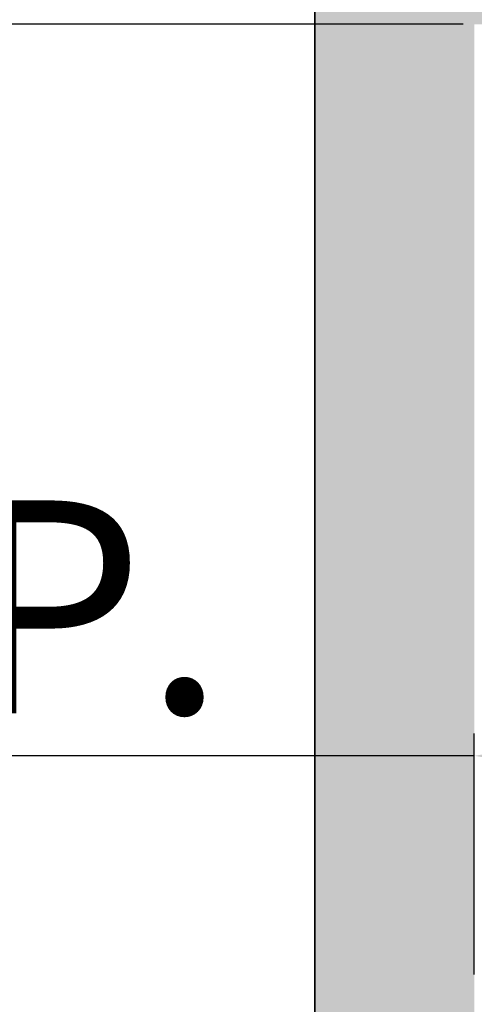
# Model space of a CAD drawing. Units: inches. Extents: x 2083 to 3317, y 1141 to 2115.
# Tile 11 of 256: x 2210 to 2236, y 1361 to 1417. Entities that reach past the tile are written whole.
import ezdxf

# ---------------------------------------------------------------- set-up
doc = ezdxf.new("R2010")
doc.units = ezdxf.units.IN
doc.layers.add('A-ANNO-DIMS', color=2, linetype='Continuous', lineweight=18)
doc.layers.add('A-WALL', color=7, linetype='Continuous', lineweight=35)
doc.layers.add('A-WALL-PATT', color=251, linetype='Continuous', lineweight=13, true_color=0x636466)
doc.styles.get("Standard").update_dxf_attribs({"font": 'arial.ttf'})
doc.dimstyles.new('ISO-25', dxfattribs={"dimtxt": 12, "dimasz": 12, "dimexe": 1.25, "dimexo": 0.625, "dimtad": 1, "dimlunit": 3, "dimtxsty": 'Standard', "dimcen": 2.5, "dimadec": 0, "dimazin": 0, "dimtfac": 1, "dimtmove": 0, "dimatfit": 3, "dimfxl": 1, "dimarcsym": 0})

# ---------------------------------------------------------------- blocks, each defined once
blk = doc.blocks.new('*D13')
at = {"layer": 'A-ANNO-DIMS', "color": 0, "lineweight": -2, "transparency": 16777216}
for p, q in [((2226.335, 1477.761), (2191.976, 1477.761)), ((2193.226, 1465.761), (2193.226, 1275.261)), ((2226.335, 1263.261), (2191.976, 1263.261))]:
    blk.add_line(p, q, dxfattribs=at)
at = {"layer": 'A-ANNO-DIMS', "color": 0, "transparency": 16777216}
for points in [[(2191.226, 1465.761), (2195.226, 1465.761), (2193.226, 1477.761)], [(2191.226, 1275.261), (2195.226, 1275.261), (2193.226, 1263.261)]]:
    blk.add_solid(points, dxfattribs=at)
at = {"layer": 'Defpoints', "color": 0, "transparency": 16777216}
for p in [(2226.96, 1477.761), (2193.226, 1263.261), (2226.96, 1263.261)]:
    blk.add_point(p, dxfattribs=at)
at = {"layer": 'A-ANNO-DIMS', "color": 0, "transparency": 16777216, "insert": (2186.474, 1370.511), "char_height": 12, "attachment_point": 5, "rotation": 90}
blk.add_mtext('17\'-10.5"', dxfattribs=at)
blk = doc.blocks.new('*D22')
at = {"layer": 'A-ANNO-DIMS', "color": 0, "lineweight": -2, "transparency": 16777216}
for p, q in [((2235.96, 1362.739), (2235.96, 1376.309)), ((2322.26, 1362.739), (2322.26, 1376.309)), ((2235.96, 1375.059), (2083.007, 1375.059)), ((2310.26, 1375.059), (2247.96, 1375.059))]:
    blk.add_line(p, q, dxfattribs=at)
at = {"layer": 'A-ANNO-DIMS', "color": 0, "transparency": 16777216}
for points in [[(2247.96, 1377.059), (2247.96, 1373.059), (2235.96, 1375.059)], [(2310.26, 1377.059), (2310.26, 1373.059), (2322.26, 1375.059)]]:
    blk.add_solid(points, dxfattribs=at)
at = {"layer": 'Defpoints', "color": 0, "transparency": 16777216}
for p in [(2235.96, 1375.059), (2235.96, 1362.114), (2322.26, 1362.114)]:
    blk.add_point(p, dxfattribs=at)
at = {"layer": 'A-ANNO-DIMS', "color": 0, "transparency": 16777216, "insert": (2153.483, 1381.889), "char_height": 12, "attachment_point": 5}
blk.add_mtext('BED 7\'-2 1/2" TYP.', dxfattribs=at)
blk = doc.blocks.new('*D30')
at = {"layer": 'A-ANNO-DIMS', "color": 0, "lineweight": -2, "transparency": 16777216}
for p, q in [((2240.018, 1445.274), (2240.018, 1448.046)), ((2254.329, 1445.274), (2254.329, 1448.046)), ((2228.018, 1446.796), (2216.018, 1446.796)), ((2240.018, 1446.796), (2254.329, 1446.796)), ((2266.329, 1446.796), (2413.765, 1446.796))]:
    blk.add_line(p, q, dxfattribs=at)
at = {"layer": 'A-ANNO-DIMS', "color": 0, "transparency": 16777216}
for points in [[(2228.018, 1448.796), (2228.018, 1444.796), (2240.018, 1446.796)], [(2266.329, 1448.796), (2266.329, 1444.796), (2254.329, 1446.796)]]:
    blk.add_solid(points, dxfattribs=at)
at = {"layer": 'Defpoints', "color": 0, "transparency": 16777216}
for p in [(2254.329, 1446.796), (2240.018, 1444.649), (2254.329, 1444.649)]:
    blk.add_point(p, dxfattribs=at)
at = {"layer": 'A-ANNO-DIMS', "color": 0, "transparency": 16777216, "insert": (2346.047, 1453.625), "char_height": 12, "attachment_point": 5}
blk.add_mtext('WC 1\'-2 1/2" TYP.', dxfattribs=at)
blk = doc.blocks.new('*D31')
at = {"layer": 'A-ANNO-DIMS', "color": 0, "lineweight": -2, "transparency": 16777216}
for p, q in [((2237.871, 1456.649), (2237.871, 1541.915)), ((2239.393, 1444.649), (2236.621, 1444.649)), ((2237.871, 1431.548), (2237.871, 1444.649)), ((2239.393, 1431.548), (2236.621, 1431.548)), ((2237.871, 1419.548), (2237.871, 1407.548))]:
    blk.add_line(p, q, dxfattribs=at)
at = {"layer": 'A-ANNO-DIMS', "color": 0, "transparency": 16777216}
for points in [[(2235.871, 1456.649), (2239.871, 1456.649), (2237.871, 1444.649)], [(2235.871, 1419.548), (2239.871, 1419.548), (2237.871, 1431.548)]]:
    blk.add_solid(points, dxfattribs=at)
at = {"layer": 'Defpoints', "color": 0, "transparency": 16777216}
for p in [(2237.871, 1444.649), (2240.018, 1444.649), (2240.018, 1431.548)]:
    blk.add_point(p, dxfattribs=at)
at = {"layer": 'A-ANNO-DIMS', "color": 0, "transparency": 16777216, "insert": (2231.217, 1505.282), "char_height": 12, "attachment_point": 5, "rotation": 90}
blk.add_mtext('1\'-1" TYP.', dxfattribs=at)
blk = doc.blocks.new('*D47')
at = {"layer": 'A-ANNO-DIMS', "color": 0, "lineweight": -2, "transparency": 16777216}
for p, q in [((2235.335, 1416.261), (2173.36, 1416.261)), ((2174.61, 1284.261), (2174.61, 1404.261)), ((2235.335, 1272.261), (2173.36, 1272.261))]:
    blk.add_line(p, q, dxfattribs=at)
at = {"layer": 'A-ANNO-DIMS', "color": 0, "transparency": 16777216}
for points in [[(2172.61, 1404.261), (2176.61, 1404.261), (2174.61, 1416.261)], [(2172.61, 1284.261), (2176.61, 1284.261), (2174.61, 1272.261)]]:
    blk.add_solid(points, dxfattribs=at)
at = {"layer": 'Defpoints', "color": 0, "transparency": 16777216}
for p in [(2174.61, 1416.261), (2235.96, 1416.261), (2235.96, 1272.261)]:
    blk.add_point(p, dxfattribs=at)
at = {"layer": 'A-ANNO-DIMS', "color": 0, "transparency": 16777216, "insert": (2167.858, 1344.261), "char_height": 12, "attachment_point": 5, "rotation": 90}
blk.add_mtext('12\'-0"', dxfattribs=at)

msp = doc.modelspace()

# ---------------------------------------------------------------- hatches: boundary and pattern name
at = {"layer": 'A-WALL-PATT'}
h = msp.add_hatch(color=256, dxfattribs=at)
h.dxf.hatch_style = 1
h.paths.add_polyline_path([(3126.96, 2020.761), (2748.96, 2020.761), (2604.96, 2020.761), (2226.96, 2020.761), (2226.96, 1702.761), (2466.96, 1702.761), (2466.96, 1582.761), (2418.96, 1582.761), (2418.96, 1477.761), (2226.96, 1477.761), (2226.96, 1263.261), (2544.96, 1263.261), (2544.96, 1411.761), (2604.96, 1411.761), (2685.96, 1411.761), (2685.96, 1420.761), (2604.96, 1420.761), (2604.96, 1573.761), (2604.96, 1702.761), (2604.96, 2011.761), (2748.96, 2011.761), (2748.96, 1702.761), (2862.96, 1702.761), (2862.96, 1621.761), (2871.96, 1621.761), (2871.96, 1702.761), (2883.96, 1702.761), (2883.96, 1706.939, -0.026459), (2883.96, 1711.761), (2757.96, 1711.761), (2757.96, 1807.761), (2787.96, 1807.761), (2787.96, 1812.261), (2757.96, 1812.261), (2757.96, 2011.761), (2877.96, 2011.761), (2877.96, 1812.261), (2847.96, 1812.261), (2847.96, 1807.761), (2889.836, 1807.761), (2889.836, 1812.261), (2882.46, 1812.261), (2882.46, 2011.761), (3117.96, 2011.761), (3117.96, 1812.261), (2937.836, 1812.261), (2937.836, 1807.761), (2995.71, 1807.761), (2995.71, 1796.118), (3000.21, 1796.118), (3000.21, 1807.761), (3117.96, 1807.761), (3117.96, 1711.761), (3000.21, 1711.761), (3000.21, 1760.118), (2998.573, 1760.118, -0.020711), (2995.71, 1760.118), (2995.71, 1711.761), (2931.96, 1711.761), (2931.96, 1702.761), (3126.96, 1702.761)])
h.paths.add_polyline_path([(2471.46, 2011.761), (2471.46, 1810.011), (2462.717, 1810.011), (2462.717, 1805.511), (2505.96, 1805.511), (2505.96, 1810.011), (2475.96, 1810.011), (2475.96, 2011.761), (2595.96, 2011.761), (2595.96, 1810.011), (2565.96, 1810.011), (2565.96, 1805.511), (2595.96, 1805.511), (2595.96, 1711.761), (2235.96, 1711.761), (2235.96, 1805.511), (2353.71, 1805.511), (2353.71, 1796.054), (2358.21, 1796.054), (2358.21, 1805.511), (2414.717, 1805.511), (2414.717, 1810.011), (2235.96, 1810.011), (2235.96, 2011.761)], flags=16)
h.paths.add_polyline_path([(2270.205, 1994.61), (2270.205, 1970.61), (2246.205, 1970.61), (2246.205, 1994.61)], flags=0)
edge = h.paths.add_edge_path(flags=0)
edge.add_ellipse((2332.027, 1899.798), major_axis=(-3.043, 3.043), ratio=0.168252, start_angle=-161.3322, end_angle=-156.3071, ccw=False)
edge.add_ellipse((2333.082, 1898.744), major_axis=(-1.055, 1.055), ratio=0.453532, start_angle=-123.371, end_angle=-94.1591)
edge = h.paths.add_edge_path(flags=0)
edge.add_ellipse((2332.027, 1968.876), major_axis=(3.043, 3.043), ratio=0.168252, start_angle=18.6678, end_angle=23.6929)
edge.add_spline(control_points=[(2332.926, 1970.691), (2332.227, 1970.336), (2330.894, 1969.659), (2328.413, 1970.932), (2327.204, 1967.749), (2324.71, 1969.956), (2322.533, 1967.012), (2320.013, 1971.296), (2317.68, 1968.158), (2316.041, 1967.102), (2315.427, 1966.81)], knot_values=[0, 0, 0, 0, 2.267059, 4.324559, 6.685584, 8.878641, 11.121502, 14.300359, 17.755284, 19.732645, 19.732645, 19.732645, 19.732645], degree=3, periodic=0)
edge.add_ellipse((2332.027, 1968.876), major_axis=(3.043, 3.043), ratio=0.168252, start_angle=18.6678, end_angle=23.6929, ccw=False)
edge.add_ellipse((2333.082, 1969.931), major_axis=(1.055, 1.055), ratio=0.453532, start_angle=56.629, end_angle=85.8409, ccw=False)
edge = h.paths.add_edge_path(flags=0)
edge.add_spline(control_points=[(2296.428, 1967.988), (2293.628, 1965.336), (2287.704, 1959.727), (2299.744, 1949.996), (2294.533, 1935.669), (2290.573, 1920.604), (2293.394, 1909.974), (2296.185, 1904.967)], knot_values=[0.099185, 0.099185, 0.099185, 0.099185, 0.345301, 0.619822, 0.982653, 1.386093, 1.810555, 1.810555, 1.810555, 1.810555], degree=3, periodic=0)
edge.add_spline(control_points=[(2296.185, 1904.967), (2297.384, 1902.619), (2298.001, 1901.949), (2298.553, 1901.468)], knot_values=[0.006246, 0.006246, 0.006246, 0.006246, 0.055476, 0.055476, 0.055476, 0.055476], degree=3, periodic=0)
edge.add_spline(control_points=[(2298.553, 1901.468), (2297.259, 1900.923), (2295.225, 1900.232), (2293.06, 1900.614), (2292.101, 1900.788), (2292.09, 1900.791)], knot_values=[0.312835, 0.312835, 0.312835, 0.312835, 0.40178, 0.474987, 0.475903, 0.475903, 0.475903, 0.475903], degree=3, periodic=0)
edge.add_arc((2292.794, 1904.664), 3.937, 215.4209, 259.6982, ccw=False)
edge.add_spline(control_points=[(2289.585, 1902.382), (2289.477, 1902.535), (2289.368, 1902.688), (2289.261, 1902.841)], knot_values=[0.102872, 0.102872, 0.102872, 0.102872, 0.116896, 0.116896, 0.116896, 0.116896], degree=3, periodic=0)
edge.add_spline(control_points=[(2289.261, 1902.841), (2288.687, 1902.55), (2287.64, 1902.02), (2285.881, 1901.874), (2283.853, 1901.504), (2281.72, 1899.711), (2278.467, 1899.493), (2276.157, 1901.883), (2272.259, 1899.804), (2267.778, 1901.843), (2262.244, 1900.184), (2257.415, 1901.782), (2254.318, 1900.726), (2253.178, 1900.337)], knot_values=[0, 0, 0, 0, 1.907977, 3.477176, 5.261074, 7.972851, 11.680248, 13.717921, 16.939592, 22.789562, 27.502503, 33.595215, 37.145618, 37.145618, 37.145618, 37.145618], degree=3, periodic=0)
edge.add_line((2253.178, 1900.337), (2250.244, 1902.841))
edge.add_line((2250.244, 1902.841), (2250.244, 1965.833))
edge.add_line((2250.244, 1965.833), (2253.178, 1968.337))
edge.add_spline(control_points=[(2253.178, 1968.337), (2254.318, 1967.948), (2257.415, 1966.892), (2262.244, 1968.49), (2267.778, 1966.831), (2271.527, 1968.537), (2273.876, 1967.828), (2274.207, 1967.728)], knot_values=[0, 0, 0, 0, 0.09018, 0.244935, 0.364644, 0.513233, 0.537855, 0.537855, 0.537855, 0.537855], degree=3, periodic=0)
edge.add_arc((2274.353, 1963.793), 3.937, 72.0511, 92.1279, ccw=False)
edge.add_arc((2281.297, 1985.23), 18.596, 252.0511, 288.5657)
edge.add_arc((2292.317, 1956.029), 12.646, 71.0268, 113.7782, ccw=False)
edge = h.paths.add_edge_path(flags=0)
edge.add_spline(control_points=[(2274.899, 1951.856), (2275.066, 1951.617), (2275.233, 1951.377), (2275.398, 1951.136)], knot_values=[1.409916, 1.409916, 1.409916, 1.409916, 1.43159, 1.43159, 1.43159, 1.43159], degree=3, periodic=0)
edge.add_spline(control_points=[(2275.398, 1951.136), (2275.792, 1950.562), (2276.179, 1949.984), (2276.546, 1949.397)], knot_values=[1.358238, 1.358238, 1.358238, 1.358238, 1.409916, 1.409916, 1.409916, 1.409916], degree=3, periodic=0)
edge.add_line((2276.546, 1949.397), (2277.437, 1947.862))
edge.add_spline(control_points=[(2277.437, 1947.862), (2276.304, 1945.673), (2274.64, 1942.427), (2274.632, 1938.094), (2272.799, 1930.852), (2274.356, 1943.897), (2275.948, 1947.923), (2276.546, 1949.397)], knot_values=[0.005632, 0.005632, 0.005632, 0.005632, 0.186014, 0.266002, 0.357087, 0.59639, 0.739732, 0.739732, 0.739732, 0.739732], degree=3, periodic=0)
edge.add_spline(control_points=[(2276.546, 1949.397), (2276.179, 1949.984), (2275.792, 1950.562), (2275.398, 1951.136)], knot_values=[1.358238, 1.358238, 1.358238, 1.358238, 1.409916, 1.409916, 1.409916, 1.409916], degree=3, periodic=0)
edge.add_spline(control_points=[(2275.398, 1951.136), (2274.943, 1950.08), (2274.208, 1948.025), (2273.935, 1944.851), (2272.469, 1937.627), (2273.466, 1945.696), (2274.701, 1951.059), (2274.899, 1951.856)], knot_values=[0.104364, 0.104364, 0.104364, 0.104364, 0.189636, 0.269624, 0.36071, 0.600013, 0.644622, 0.644622, 0.644622, 0.644622], degree=3, periodic=0)
h.paths.add_polyline_path([(2269.168, 1963.128, -0.357527), (2268.171, 1960.976, -0.092561), (2268.171, 1939.436, -0.357527), (2269.168, 1937.285, -0.357527), (2267.016, 1938.282, -0.164785), (2254.686, 1938.282, -0.357527), (2252.534, 1937.285, -0.357527), (2253.531, 1939.436, -0.092561), (2253.531, 1960.976, -0.357527), (2252.534, 1963.128, -0.357527), (2254.686, 1962.131, -0.164785), (2267.016, 1962.131, -0.357527)], flags=0)
h.paths.add_polyline_path([(2248.874, 1967.802), (2248.874, 1957.028), (2249.458, 1957.028), (2249.458, 1911.647), (2248.874, 1911.647), (2248.874, 1900.873), (2246.512, 1900.873, 0.197327), (2244.15, 1902.457), (2244.15, 1966.218, 0.197327), (2246.512, 1967.802)], flags=0)
h.paths.add_polyline_path([(2269.168, 1931.389, -0.357527), (2268.171, 1929.238, -0.092561), (2268.171, 1907.698, -0.357527), (2269.168, 1905.547, -0.357527), (2267.016, 1906.544, -0.164785), (2254.686, 1906.544, -0.357527), (2252.534, 1905.547, -0.357527), (2253.531, 1907.698, -0.092561), (2253.531, 1929.238, -0.357527), (2252.534, 1931.389, -0.357527), (2254.686, 1930.392, -0.164785), (2267.016, 1930.392, -0.357527)], flags=0)
edge = h.paths.add_edge_path(flags=0)
edge.add_spline(control_points=[(2276.197, 1906.724), (2276.168, 1909.029), (2276.114, 1913.372), (2270.598, 1924.925), (2273.905, 1919.013), (2275.922, 1916.262), (2275.475, 1912.402), (2277.258, 1910.381), (2276.696, 1908.225), (2276.646, 1906.813), (2276.618, 1906.008)], knot_values=[0, 0, 0, 0, 8.61026, 16.221274, 18.843057, 23.804898, 27.440828, 29.356102, 31.203478, 33.650687, 33.650687, 33.650687, 33.650687], degree=3, periodic=0)
edge.add_spline(control_points=[(2276.618, 1906.008), (2276.623, 1905.624), (2276.498, 1904.629), (2275.442, 1903.855), (2274.937, 1903.08), (2274.859, 1902.841)], knot_values=[0.156488, 0.156488, 0.156488, 0.156488, 0.184398, 0.231376, 0.250598, 0.250598, 0.250598, 0.250598], degree=3, periodic=0)
edge.add_line((2274.859, 1902.841), (2276.506, 1902.841))
edge.add_spline(control_points=[(2276.506, 1902.841), (2276.788, 1903.085), (2277.665, 1904.125), (2278.25, 1904.341), (2277.654, 1908.527), (2278.156, 1906.228), (2278.1, 1905.286), (2278.847, 1904.069), (2277.857, 1903.415), (2277.874, 1902.991), (2277.904, 1902.841)], knot_values=[0.059574, 0.059574, 0.059574, 0.059574, 0.080753, 0.103741, 0.16972, 0.176036, 0.207137, 0.240474, 0.262341, 0.27366, 0.27366, 0.27366, 0.27366], degree=3, periodic=0)
edge.add_line((2277.904, 1902.841), (2280.03, 1902.841))
edge.add_spline(control_points=[(2280.03, 1902.841), (2279.888, 1903.088), (2279.499, 1903.982), (2280.152, 1905.939), (2278.104, 1909.658), (2279.762, 1907.185), (2280.328, 1904.875), (2280.485, 1903.49), (2281.463, 1903.249), (2281.758, 1902.936), (2281.834, 1902.841)], knot_values=[0.013856, 0.013856, 0.013856, 0.013856, 0.034874, 0.088867, 0.107879, 0.126738, 0.158714, 0.193757, 0.217487, 0.226722, 0.226722, 0.226722, 0.226722], degree=3, periodic=0)
edge.add_spline(control_points=[(2281.834, 1902.841), (2281.788, 1902.827), (2281.647, 1902.783), (2281.396, 1902.859), (2281.088, 1902.985), (2280.721, 1903.061), (2280.333, 1903.026), (2280.125, 1902.899), (2280.03, 1902.841)], knot_values=[0, 0, 0, 0, 0.14413, 0.435517, 0.749276, 1.153046, 1.548371, 1.878348, 1.878348, 1.878348, 1.878348], degree=3, periodic=0)
edge.add_line((2280.03, 1902.841), (2277.904, 1902.841))
edge.add_spline(control_points=[(2277.904, 1902.841), (2277.893, 1902.796), (2277.865, 1902.68), (2277.607, 1902.687), (2277.274, 1902.801), (2276.838, 1902.62), (2276.584, 1902.789), (2276.506, 1902.841)], knot_values=[0, 0, 0, 0, 0.127189, 0.326199, 0.628009, 1.24357, 1.515331, 1.515331, 1.515331, 1.515331], degree=3, periodic=0)
edge.add_line((2276.506, 1902.841), (2274.859, 1902.841))
edge.add_spline(control_points=[(2274.859, 1902.841), (2274.814, 1902.899), (2274.725, 1903.013), (2274.493, 1903.119), (2274.244, 1902.961), (2273.937, 1903.185), (2273.614, 1902.983), (2273.408, 1902.883), (2273.322, 1902.841)], knot_values=[0, 0, 0, 0, 0.21843, 0.436957, 0.687977, 0.990379, 1.398396, 1.69185, 1.69185, 1.69185, 1.69185], degree=3, periodic=0)
edge.add_spline(control_points=[(2273.322, 1902.841), (2273.617, 1903.446), (2274.274, 1904.538), (2276.027, 1904.574), (2276.207, 1906.584), (2276.197, 1906.724)], knot_values=[0.012227, 0.012227, 0.012227, 0.012227, 0.059472, 0.106218, 0.134458, 0.134458, 0.134458, 0.134458], degree=3, periodic=0)
h.paths.add_polyline_path([(2270.776, 1897.79), (2270.776, 1873.79), (2246.776, 1873.79), (2246.776, 1897.79)], flags=0)
h.paths.add_polyline_path([(2353.71, 1760.005), (2353.71, 1760.054), (2358.21, 1760.054, -0.033729)], flags=0)
h.paths.add_polyline_path([(2321.819, 1737.529), (2341.995, 1737.529, -0.414214), (2343.203, 1736.321), (2343.203, 1721.021, -0.414214), (2341.995, 1719.813), (2321.819, 1719.813, -0.414214), (2320.611, 1721.021), (2320.611, 1736.321, -0.414214)], flags=0)
h.paths.add_polyline_path([(2324.235, 1736.321), (2339.579, 1736.321, -0.414214), (2341.995, 1733.905), (2341.995, 1725.45, -0.414214), (2339.579, 1723.034), (2333.681, 1723.034), (2333.845, 1722.045, -0.870646), (2335.425, 1721.826, -0.767327), (2333.923, 1721.423), (2331.291, 1721.423, -0.767327), (2329.788, 1721.826, -0.870646), (2331.368, 1722.045), (2331.533, 1723.034), (2324.235, 1723.034, -0.414214), (2321.819, 1725.45), (2321.819, 1733.905, -0.414214)], flags=0)
h.paths.add_polyline_path([(2570.484, 1928.615), (2589.684, 1928.615), (2590.169, 1928.615), (2590.169, 1904.993), (2570.484, 1904.993)], flags=0)
h.paths.add_polyline_path([(2574.447, 1927.264, -1), (2572.829, 1927.264, -1)], flags=0)
h.paths.add_polyline_path([(2573.09, 1926.941), (2573.925, 1927.776), (2574.148, 1927.553), (2573.313, 1926.718)], flags=0)
h.paths.add_polyline_path([(2578.779, 1919.73, -1), (2571.592, 1919.73, -1)], flags=0)
h.paths.add_polyline_path([(2578.385, 1919.73, -1), (2571.985, 1919.73, -1)], flags=0)
h.paths.add_polyline_path([(2331.596, 1729.476, -1), (2333.618, 1729.476, -1)], flags=0)
h.paths.add_polyline_path([(2578.034, 1927.264, -1), (2576.416, 1927.264, -1)], flags=0)
h.paths.add_polyline_path([(2576.689, 1927.531), (2576.912, 1927.754), (2577.747, 1926.919), (2577.524, 1926.696)], flags=0)
h.paths.add_polyline_path([(2578.139, 1909.86, -1), (2572.232, 1909.86, -1)], flags=0)
h.paths.add_polyline_path([(2577.745, 1909.86, -1), (2572.625, 1909.86, -1)], flags=0)
h.paths.add_polyline_path([(2583.798, 1927.264, -1), (2582.179, 1927.264, -1)], flags=0)
h.paths.add_polyline_path([(2582.719, 1927.754), (2583.554, 1926.919), (2583.331, 1926.696), (2582.496, 1927.531)], flags=0)
h.paths.add_polyline_path([(2582.496, 1927.531), (2582.719, 1927.754), (2583.554, 1926.919), (2583.331, 1926.696)], flags=0)
h.paths.add_polyline_path([(2587.739, 1920.53, -1), (2581.832, 1920.53, -1)], flags=0)
h.paths.add_polyline_path([(2587.345, 1920.53, -1), (2582.225, 1920.53, -1)], flags=0)
h.paths.add_polyline_path([(2587.385, 1927.264, -1), (2585.766, 1927.264, -1)], flags=0)
h.paths.add_polyline_path([(2586.082, 1926.98), (2586.917, 1927.815), (2587.14, 1927.593), (2586.305, 1926.758)], flags=0)
h.paths.add_polyline_path([(2588.379, 1910.66, -1), (2581.192, 1910.66, -1)], flags=0)
h.paths.add_polyline_path([(2587.985, 1910.66, -1), (2581.585, 1910.66, -1)], flags=0)
h.paths.add_polyline_path([(2417.168, 1729.478), (2437.344, 1729.478, -0.414214), (2438.552, 1728.27), (2438.552, 1712.969, -0.414214), (2437.344, 1711.761), (2417.168, 1711.761, -0.414214), (2415.96, 1712.969), (2415.96, 1728.27, -0.414214)], flags=0)
h.paths.add_polyline_path([(2419.584, 1728.27), (2434.928, 1728.27, -0.414214), (2437.344, 1725.854), (2437.344, 1717.398, -0.414214), (2434.928, 1714.983), (2429.029, 1714.983), (2429.194, 1713.994, -0.870646), (2430.774, 1713.775, -0.767327), (2429.271, 1713.372), (2426.64, 1713.372, -0.767327), (2425.137, 1713.775, -0.870646), (2426.717, 1713.994), (2426.882, 1714.983), (2419.584, 1714.983, -0.414214), (2417.168, 1717.398), (2417.168, 1725.854, -0.414214)], flags=0)
h.paths.add_polyline_path([(2419.584, 1728.27), (2434.928, 1728.27, -0.414214), (2437.344, 1725.854), (2437.344, 1717.398, -0.414214), (2434.928, 1714.983), (2429.029, 1714.983), (2428.358, 1719.009), (2427.553, 1719.009), (2426.882, 1714.983), (2419.584, 1714.983, -0.414214), (2417.168, 1717.398), (2417.168, 1725.854, -0.414214)], flags=0)
h.paths.add_polyline_path([(2426.944, 1721.425, -1), (2428.967, 1721.425, -1)], flags=0)
h.paths.add_polyline_path([(2475.96, 1702.761), (2595.96, 1702.761), (2595.96, 1582.761), (2475.96, 1582.761)], flags=16)
h.paths.add_polyline_path([(2427.96, 1573.761), (2595.96, 1573.761), (2595.96, 1468.761), (2595.96, 1420.761), (2384.46, 1420.761), (2384.46, 1468.761), (2427.96, 1468.761)], flags=16)
h.paths.add_polyline_path([(2379.96, 1468.761), (2379.96, 1420.761), (2235.96, 1420.761), (2235.96, 1468.761)], flags=16)
h.paths.add_polyline_path([(2317.816, 1466.696), (2337.992, 1466.696, -0.414214), (2339.2, 1465.488), (2339.2, 1450.187, -0.414214), (2337.992, 1448.979), (2317.816, 1448.979, -0.414214), (2316.608, 1450.187), (2316.608, 1465.488, -0.414214)], flags=0)
h.paths.add_polyline_path([(2320.232, 1465.488), (2335.576, 1465.488, -0.414214), (2337.992, 1463.072), (2337.992, 1454.616, -0.414214), (2335.576, 1452.2), (2329.677, 1452.2), (2329.842, 1451.212, -0.870646), (2331.422, 1450.992, -0.767327), (2329.92, 1450.59), (2327.288, 1450.59, -0.767327), (2325.785, 1450.992, -0.870646), (2327.365, 1451.212), (2327.53, 1452.2), (2320.232, 1452.2, -0.414214), (2317.816, 1454.616), (2317.816, 1463.072, -0.414214)], flags=0)
h.paths.add_polyline_path([(2320.232, 1465.488), (2335.576, 1465.488, -0.414214), (2337.992, 1463.072), (2337.992, 1454.616, -0.414214), (2335.576, 1452.2), (2329.677, 1452.2), (2329.006, 1456.227), (2328.201, 1456.227), (2327.53, 1452.2), (2320.232, 1452.2, -0.414214), (2317.816, 1454.616), (2317.816, 1463.072, -0.414214)], flags=0)
h.paths.add_polyline_path([(2327.593, 1458.643, -1), (2329.615, 1458.643, -1)], flags=0)
h.paths.add_polyline_path([(2244.412, 1433.34), (2241.921, 1433.34, -0.414214), (2240.018, 1435.244), (2240.018, 1440.953, -0.414211), (2241.921, 1442.856), (2244.412, 1442.856, -1.976472)], flags=0)
h.paths.add_polyline_path([(2245.357, 1434.398, -0.414214), (2245.357, 1441.799, -2.144098)], flags=0)
h.paths.add_polyline_path([(2535.96, 1416.261), (2535.96, 1272.261), (2235.96, 1272.261), (2235.96, 1416.261)], flags=16)
h.paths.add_polyline_path([(2260.12, 1384.293), (2260.12, 1362.039), (2237.865, 1362.039), (2237.865, 1384.293)], flags=0)
edge = h.paths.add_edge_path(flags=0)
edge.add_line((2318.252, 1362.093), (2318.146, 1362.001))
edge.add_ellipse((2317.445, 1360.431), major_axis=(2.822, 2.822), ratio=0.168252, start_angle=18.6678, end_angle=20.9481, ccw=False)
edge.add_ellipse((2318.423, 1361.409), major_axis=(0.978, 0.978), ratio=0.453532, start_angle=56.629, end_angle=70.2262, ccw=False)
edge = h.paths.add_edge_path(flags=0)
edge.add_line((2319.107, 1295.571), (2319.015, 1295.677))
edge.add_ellipse((2317.445, 1296.378), major_axis=(-2.822, 2.822), ratio=0.168252, start_angle=-161.3322, end_angle=-159.0519, ccw=False)
edge.add_ellipse((2318.423, 1295.4), major_axis=(-0.978, 0.978), ratio=0.453532, start_angle=-123.371, end_angle=-109.7738)
edge = h.paths.add_edge_path(flags=0)
edge.add_spline(control_points=[(2284.21, 1301.17), (2284.581, 1300.445), (2284.891, 1299.892), (2285.16, 1299.461)], knot_values=[0.039066, 0.039066, 0.039066, 0.039066, 0.055476, 0.055476, 0.055476, 0.055476], degree=3, periodic=0)
edge.add_line((2285.16, 1299.461), (2284.21, 1301.17))
edge = h.paths.add_edge_path(flags=0)
edge.add_line((2280.412, 1297.298), (2283.37, 1297.036))
edge.add_line((2283.37, 1297.036), (2286.406, 1297.926))
edge.add_spline(control_points=[(2286.406, 1297.926), (2285.305, 1297.463), (2284.345, 1297.129), (2283.37, 1297.036)], knot_values=[0.394369, 0.394369, 0.394369, 0.394369, 0.475903, 0.475903, 0.475903, 0.475903], degree=3, periodic=0)
edge.add_spline(control_points=[(2283.37, 1297.036), (2283.281, 1297.028), (2282.316, 1296.957), (2281.313, 1297.134), (2280.423, 1297.296), (2280.412, 1297.298)], knot_values=[0.312835, 0.312835, 0.312835, 0.312835, 0.320246, 0.393453, 0.394369, 0.394369, 0.394369, 0.394369], degree=3, periodic=0)
edge = h.paths.add_edge_path(flags=0)
edge.add_line((2284.436, 1359.607), (2280.446, 1355.328))
edge.add_line((2280.446, 1355.328), (2279.58, 1351.018))
edge.add_line((2279.58, 1351.018), (2282.413, 1346.58))
edge.add_spline(control_points=[(2282.413, 1346.58), (2283.153, 1345.589), (2284.253, 1344.029), (2284.801, 1342.387), (2284.935, 1341.806)], knot_values=[1.240098, 1.240098, 1.240098, 1.240098, 1.332892, 1.382712, 1.382712, 1.382712, 1.382712], degree=3, periodic=0)
edge.add_spline(control_points=[(2284.935, 1341.806), (2285.319, 1340.141), (2285.233, 1338.409), (2284.91, 1336.654)], knot_values=[1.097484, 1.097484, 1.097484, 1.097484, 1.240098, 1.240098, 1.240098, 1.240098], degree=3, periodic=0)
edge.add_spline(control_points=[(2284.91, 1336.654), (2284.587, 1334.899), (2284.027, 1333.12), (2283.463, 1331.361)], knot_values=[0.95487, 0.95487, 0.95487, 0.95487, 1.097484, 1.097484, 1.097484, 1.097484], degree=3, periodic=0)
edge.add_line((2283.463, 1331.361), (2281.89, 1326.153))
edge.add_line((2281.89, 1326.153), (2280.756, 1321.056))
edge.add_line((2280.756, 1321.056), (2280.299, 1316.002))
edge.add_line((2280.299, 1316.002), (2280.716, 1310.95))
edge.add_line((2280.716, 1310.95), (2282.028, 1305.972))
edge.add_line((2282.028, 1305.972), (2284.21, 1301.17))
edge.add_spline(control_points=[(2284.21, 1301.17), (2283.341, 1302.73), (2282.612, 1304.336), (2282.028, 1305.972)], knot_values=[0.099185, 0.099185, 0.099185, 0.099185, 0.241799, 0.241799, 0.241799, 0.241799], degree=3, periodic=0)
edge.add_spline(control_points=[(2282.028, 1305.972), (2281.444, 1307.608), (2281.005, 1309.273), (2280.716, 1310.95)], knot_values=[0.241799, 0.241799, 0.241799, 0.241799, 0.384413, 0.384413, 0.384413, 0.384413], degree=3, periodic=0)
edge.add_spline(control_points=[(2280.716, 1310.95), (2280.433, 1312.588), (2280.289, 1314.277), (2280.299, 1315.962), (2280.299, 1316.002)], knot_values=[0.384413, 0.384413, 0.384413, 0.384413, 0.523647, 0.527028, 0.527028, 0.527028, 0.527028], degree=3, periodic=0)
edge.add_spline(control_points=[(2280.299, 1316.002), (2280.312, 1317.687), (2280.478, 1319.368), (2280.756, 1321.056)], knot_values=[0.527028, 0.527028, 0.527028, 0.527028, 0.669642, 0.669642, 0.669642, 0.669642], degree=3, periodic=0)
edge.add_spline(control_points=[(2280.756, 1321.056), (2281.035, 1322.744), (2281.426, 1324.44), (2281.89, 1326.153)], knot_values=[0.669642, 0.669642, 0.669642, 0.669642, 0.812256, 0.812256, 0.812256, 0.812256], degree=3, periodic=0)
edge.add_spline(control_points=[(2281.89, 1326.153), (2282.264, 1327.533), (2282.788, 1329.262), (2283.353, 1331.018), (2283.463, 1331.361)], knot_values=[0.812256, 0.812256, 0.812256, 0.812256, 0.927087, 0.95487, 0.95487, 0.95487, 0.95487], degree=3, periodic=0)
edge.add_line((2283.463, 1331.361), (2284.91, 1336.654))
edge.add_line((2284.91, 1336.654), (2284.935, 1341.806))
edge.add_line((2284.935, 1341.806), (2282.413, 1346.58))
edge.add_spline(control_points=[(2282.413, 1346.58), (2281.275, 1348.104), (2280.078, 1349.57), (2279.58, 1351.018)], knot_values=[1.382712, 1.382712, 1.382712, 1.382712, 1.525326, 1.525326, 1.525326, 1.525326], degree=3, periodic=0)
edge.add_spline(control_points=[(2279.58, 1351.018), (2279.443, 1351.415), (2279.136, 1352.857), (2279.735, 1354.29), (2280.446, 1355.328)], knot_values=[1.525326, 1.525326, 1.525326, 1.525326, 1.564439, 1.667941, 1.667941, 1.667941, 1.667941], degree=3, periodic=0)
edge.add_spline(control_points=[(2280.446, 1355.328), (2281.426, 1356.758), (2282.931, 1358.183), (2284.436, 1359.607)], knot_values=[1.667941, 1.667941, 1.667941, 1.667941, 1.810555, 1.810555, 1.810555, 1.810555], degree=3, periodic=0)
edge.add_arc((2280.623, 1348.518), 11.726, 71.0268, 113.7782)
edge.add_arc((2270.405, 1375.595), 17.244, 252.0511, 288.5657, ccw=False)
edge.add_arc((2263.966, 1355.718), 3.651, 72.0511, 92.1279)
edge.add_arc((2263.966, 1355.718), 3.651, 92.1279, 177.9851)
edge.add_spline(control_points=[(2260.318, 1355.846), (2260.26, 1354.221), (2260.551, 1350.187), (2262.999, 1346.766), (2264.473, 1344.649)], knot_values=[1.43159, 1.43159, 1.43159, 1.43159, 1.564144, 1.770695, 1.770695, 1.770695, 1.770695], degree=3, periodic=0)
edge.add_line((2264.473, 1344.649), (2264.936, 1343.983))
edge.add_spline(control_points=[(2263.801, 1340.248), (2263.843, 1340.514), (2264.067, 1341.756), (2264.513, 1343.002), (2264.935, 1343.981)], knot_values=[0.53657, 0.53657, 0.53657, 0.53657, 0.559349, 0.644622, 0.644622, 0.644622, 0.644622], degree=3, periodic=0)
edge.add_spline(control_points=[(2264.935, 1343.981), (2265.118, 1343.715), (2265.299, 1343.448), (2265.477, 1343.179)], knot_values=[1.384077, 1.384077, 1.384077, 1.384077, 1.409916, 1.409916, 1.409916, 1.409916], degree=3, periodic=0)
edge.add_spline(control_points=[(2265.477, 1343.179), (2265.655, 1342.911), (2265.829, 1342.641), (2265.999, 1342.369)], knot_values=[1.358238, 1.358238, 1.358238, 1.358238, 1.384077, 1.384077, 1.384077, 1.384077], degree=3, periodic=0)
edge.add_line((2265.999, 1342.369), (2266.826, 1340.946))
edge.add_spline(control_points=[(2266.826, 1340.946), (2268.894, 1337.09), (2271.398, 1325.843), (2270.516, 1310.569), (2275.919, 1301.861), (2277.79, 1299.199)], knot_values=[0.116896, 0.116896, 0.116896, 0.116896, 0.472987, 1.050969, 1.313793, 1.313793, 1.313793, 1.313793], degree=3, periodic=0)
edge.add_spline(control_points=[(2277.79, 1299.199), (2277.839, 1299.128), (2277.889, 1299.057), (2277.94, 1298.987)], knot_values=[0.109884, 0.109884, 0.109884, 0.109884, 0.116896, 0.116896, 0.116896, 0.116896], degree=3, periodic=0)
edge.add_line((2277.94, 1298.987), (2277.789, 1299.199))
edge.add_spline(control_points=[(2277.789, 1299.199), (2277.257, 1298.929), (2276.286, 1298.438), (2275.039, 1298.334), (2274.383, 1298.239), (2274.215, 1298.209)], knot_values=[33.12187, 33.12187, 33.12187, 33.12187, 35.029056, 36.598255, 37.144827, 37.144827, 37.144827, 37.144827], degree=3, periodic=0)
edge.add_line((2274.215, 1298.209), (2273.073, 1297.893))
edge.add_spline(control_points=[(2273.073, 1297.893), (2272.323, 1297.58), (2271.039, 1296.511), (2269.248, 1296.226), (2268.423, 1296.375)], knot_values=[26.532584, 26.532584, 26.532584, 26.532584, 29.198919, 31.839101, 31.839101, 31.839101, 31.839101], degree=3, periodic=0)
edge.add_line((2268.423, 1296.375), (2263.879, 1297.458))
edge.add_spline(control_points=[(2263.879, 1297.458), (2263.556, 1297.359), (2261.86, 1296.839), (2260.239, 1297.282), (2258.933, 1297.516)], knot_values=[15.919551, 15.919551, 15.919551, 15.919551, 16.939592, 21.226067, 21.226067, 21.226067, 21.226067], degree=3, periodic=0)
edge.add_line((2258.933, 1297.516), (2254.055, 1297.329))
edge.add_spline(control_points=[(2254.055, 1297.329), (2253.756, 1297.296), (2252.114, 1297.165), (2250.462, 1297.544), (2249.13, 1297.668)], knot_values=[5.306517, 5.306517, 5.306517, 5.306517, 6.276435, 10.613034, 10.613034, 10.613034, 10.613034], degree=3, periodic=0)
edge.add_line((2249.13, 1297.668), (2244.332, 1296.878))
edge.add_line((2244.332, 1296.878), (2241.611, 1299.199))
edge.add_line((2241.611, 1299.199), (2241.611, 1357.609))
edge.add_line((2241.611, 1357.609), (2244.332, 1359.931))
edge.add_line((2244.332, 1359.931), (2252.729, 1359.543))
edge.add_spline(control_points=[(2252.729, 1359.543), (2252.871, 1359.546), (2253.306, 1359.548), (2253.74, 1359.514), (2254.032, 1359.482)], knot_values=[0.233291, 0.233291, 0.233291, 0.233291, 0.244935, 0.268927, 0.268927, 0.268927, 0.268927], degree=3, periodic=0)
edge.add_line((2254.032, 1359.482), (2259.587, 1359.416))
edge.add_spline(control_points=[(2259.587, 1359.416), (2260.677, 1359.629), (2262.073, 1359.897), (2263.524, 1359.459), (2263.83, 1359.366)], knot_values=[0.422516, 0.422516, 0.422516, 0.422516, 0.513233, 0.537855, 0.537855, 0.537855, 0.537855], degree=3, periodic=0)
edge.add_arc((2263.966, 1355.718), 3.651, 72.0511, 92.1279, ccw=False)
edge.add_arc((2270.405, 1375.595), 17.244, 252.0511, 288.5657)
edge.add_arc((2280.623, 1348.518), 11.726, 71.0268, 113.7782, ccw=False)
h.paths.add_polyline_path([(2240.341, 1359.435), (2240.341, 1349.444), (2240.882, 1349.444), (2240.882, 1307.365), (2240.341, 1307.365), (2240.341, 1297.374), (2238.15, 1297.374, 0.197327), (2235.96, 1298.843), (2235.96, 1357.966, 0.197327), (2238.15, 1359.435)], flags=0)
h.paths.add_polyline_path([(2259.158, 1355.101, -0.357527), (2258.233, 1353.106, -0.092561), (2258.233, 1333.133, -0.357527), (2259.158, 1331.138, -0.357527), (2257.163, 1332.062, -0.164785), (2245.729, 1332.062, -0.357527), (2243.735, 1331.138, -0.357527), (2244.659, 1333.133, -0.092561), (2244.659, 1353.106, -0.357527), (2243.735, 1355.101, -0.357527), (2245.729, 1354.176, -0.164785), (2257.163, 1354.176, -0.357527)], flags=0)
edge = h.paths.add_edge_path(flags=0)
edge.add_line((2265.999, 1342.369), (2266.826, 1340.946))
edge.add_line((2266.826, 1340.946), (2265.308, 1337.814))
edge.add_line((2265.308, 1337.814), (2264.358, 1334.653))
edge.add_line((2264.358, 1334.653), (2264.262, 1333.8))
edge.add_spline(control_points=[(2264.262, 1333.8), (2264.208, 1333.187), (2264.162, 1332.366), (2264.007, 1331.414), (2263.969, 1331.202)], knot_values=[0.464444, 0.464444, 0.464444, 0.464444, 0.516691, 0.531608, 0.531608, 0.531608, 0.531608], degree=3, periodic=0)
edge.add_spline(control_points=[(2263.969, 1331.202), (2263.775, 1330.119), (2263.424, 1328.791), (2263.257, 1328.531), (2263.234, 1328.515)], knot_values=[0.372682, 0.372682, 0.372682, 0.372682, 0.44885, 0.464444, 0.464444, 0.464444, 0.464444], degree=3, periodic=0)
edge.add_spline(control_points=[(2263.234, 1328.515), (2263.096, 1328.42), (2263.131, 1329.301), (2263.275, 1330.616)], knot_values=[0.280919, 0.280919, 0.280919, 0.280919, 0.372682, 0.372682, 0.372682, 0.372682], degree=3, periodic=0)
edge.add_spline(control_points=[(2263.275, 1330.616), (2263.419, 1331.93), (2263.672, 1333.677), (2263.97, 1335.315)], knot_values=[0.189157, 0.189157, 0.189157, 0.189157, 0.280919, 0.280919, 0.280919, 0.280919], degree=3, periodic=0)
edge.add_spline(control_points=[(2263.97, 1335.315), (2264.1, 1336.032), (2264.419, 1337.622), (2264.755, 1338.864), (2264.947, 1339.491)], knot_values=[0.097394, 0.097394, 0.097394, 0.097394, 0.137578, 0.189157, 0.189157, 0.189157, 0.189157], degree=3, periodic=0)
edge.add_spline(control_points=[(2264.947, 1339.491), (2265.29, 1340.606), (2265.644, 1341.494), (2265.999, 1342.369)], knot_values=[0.005632, 0.005632, 0.005632, 0.005632, 0.097394, 0.097394, 0.097394, 0.097394], degree=3, periodic=0)
h.paths.add_polyline_path([(2259.158, 1325.671, -0.357527), (2258.233, 1323.676, -0.092561), (2258.233, 1303.703, -0.357527), (2259.158, 1301.708, -0.357527), (2257.163, 1302.633, -0.164785), (2245.729, 1302.633, -0.357527), (2243.735, 1301.708, -0.357527), (2244.659, 1303.703, -0.092561), (2244.659, 1323.676, -0.357527), (2243.735, 1325.671, -0.357527), (2245.729, 1324.747, -0.164785), (2257.163, 1324.747, -0.357527)], flags=0)
edge = h.paths.add_edge_path(flags=0)
edge.add_spline(control_points=[(2261.709, 1317.311), (2261.679, 1317.418), (2261.762, 1317.389), (2262.491, 1316.09), (2262.962, 1315.301)], knot_values=[14.955861, 14.955861, 14.955861, 14.955861, 16.221274, 18.694826, 18.694826, 18.694826, 18.694826], degree=3, periodic=0)
edge.add_spline(control_points=[(2262.962, 1315.301), (2262.99, 1315.254), (2263.702, 1314.067), (2264.349, 1313.127), (2264.73, 1312.164)], knot_values=[18.694826, 18.694826, 18.694826, 18.694826, 18.843057, 22.433791, 22.433791, 22.433791, 22.433791], degree=3, periodic=0)
edge.add_spline(control_points=[(2264.73, 1312.164), (2264.876, 1311.796), (2265.177, 1310.77), (2265.143, 1309.559), (2265.248, 1308.824)], knot_values=[22.433791, 22.433791, 22.433791, 22.433791, 23.804898, 26.172756, 26.172756, 26.172756, 26.172756], degree=3, periodic=0)
edge.add_line((2265.248, 1308.824), (2265.851, 1307.172))
edge.add_spline(control_points=[(2265.851, 1307.172), (2266.065, 1306.822), (2266.384, 1306.332), (2266.424, 1305.781), (2266.42, 1305.611)], knot_values=[28.062562, 28.062562, 28.062562, 28.062562, 29.356102, 29.911721, 29.911721, 29.911721, 29.911721], degree=3, periodic=0)
edge.add_spline(control_points=[(2266.42, 1305.611), (2266.416, 1305.433), (2266.394, 1305.25), (2266.365, 1305.066)], knot_values=[29.911721, 29.911721, 29.911721, 29.911721, 30.497837, 30.497837, 30.497837, 30.497837], degree=3, periodic=0)
edge.add_line((2266.365, 1305.066), (2266.066, 1302.136))
edge.add_spline(control_points=[(2266.066, 1302.136), (2266.071, 1301.78), (2265.998, 1301.2), (2265.663, 1300.759), (2265.509, 1300.586)], knot_values=[0.156488, 0.156488, 0.156488, 0.156488, 0.184398, 0.203543, 0.203543, 0.203543, 0.203543], degree=3, periodic=0)
edge.add_line((2265.509, 1300.586), (2264.435, 1299.199))
edge.add_line((2264.435, 1299.199), (2265.962, 1299.199))
edge.add_line((2265.962, 1299.199), (2267.336, 1301.175))
edge.add_line((2267.336, 1301.175), (2267.312, 1301.986))
edge.add_spline(control_points=[(2267.312, 1301.986), (2267.261, 1302.862), (2267.16, 1303.737), (2267.271, 1303.326)], knot_values=[0.126229, 0.126229, 0.126229, 0.126229, 0.166617, 0.166617, 0.166617, 0.166617], degree=3, periodic=0)
edge.add_spline(control_points=[(2267.271, 1303.326), (2267.28, 1303.294), (2267.31, 1303.175), (2267.373, 1302.884), (2267.406, 1302.683), (2267.418, 1302.601)], knot_values=[0.166617, 0.166617, 0.166617, 0.166617, 0.16972, 0.176036, 0.180765, 0.180765, 0.180765, 0.180765], degree=3, periodic=0)
edge.add_spline(control_points=[(2267.744, 1300.988), (2267.688, 1301.151), (2267.481, 1301.657), (2267.484, 1302.145), (2267.418, 1302.601)], knot_values=[0.180765, 0.180765, 0.180765, 0.180765, 0.193767, 0.220139, 0.220139, 0.220139, 0.220139], degree=3, periodic=0)
edge.add_line((2267.418, 1302.601), (2267.744, 1300.988))
edge.add_spline(control_points=[(2267.744, 1300.988), (2267.832, 1300.732), (2267.932, 1300.31), (2267.555, 1299.975), (2267.429, 1299.829)], knot_values=[0.220139, 0.220139, 0.220139, 0.220139, 0.240474, 0.25489, 0.25489, 0.25489, 0.25489], degree=3, periodic=0)
edge.add_line((2267.429, 1299.829), (2267.258, 1299.199))
edge.add_line((2267.258, 1299.199), (2269.23, 1299.199))
edge.add_spline(control_points=[(2269.23, 1299.199), (2269.099, 1299.429), (2268.843, 1300.016), (2269.012, 1300.916), (2268.947, 1301.661)], knot_values=[0.013856, 0.013856, 0.013856, 0.013856, 0.034874, 0.067073, 0.067073, 0.067073, 0.067073], degree=3, periodic=0)
edge.add_line((2268.947, 1301.661), (2268.432, 1303.603))
edge.add_spline(control_points=[(2268.432, 1303.603), (2268.176, 1304.192), (2267.596, 1305.251), (2268.041, 1304.623), (2268.251, 1304.282)], knot_values=[0.090155, 0.090155, 0.090155, 0.090155, 0.107879, 0.120289, 0.120289, 0.120289, 0.120289], degree=3, periodic=0)
edge.add_spline(control_points=[(2268.251, 1304.282), (2268.361, 1304.105), (2269.058, 1302.918), (2269.383, 1301.59), (2269.521, 1300.776), (2269.575, 1300.556)], knot_values=[0.120289, 0.120289, 0.120289, 0.120289, 0.126738, 0.158714, 0.173506, 0.173506, 0.173506, 0.173506], degree=3, periodic=0)
edge.add_line((2269.575, 1300.556), (2270.686, 1299.421))
edge.add_spline(control_points=[(2270.686, 1299.421), (2270.767, 1299.357), (2270.838, 1299.281), (2270.903, 1299.199)], knot_values=[0.21816, 0.21816, 0.21816, 0.21816, 0.226722, 0.226722, 0.226722, 0.226722], degree=3, periodic=0)
edge.add_line((2270.937, 1299.193), (2270.903, 1299.199))
edge.add_spline(control_points=[(2270.903, 1299.199), (2270.86, 1299.186), (2270.73, 1299.146), (2270.496, 1299.216), (2270.272, 1299.308), (2270.121, 1299.348), (2270.063, 1299.36)], knot_values=[0.939174, 0.939174, 0.939174, 0.939174, 1.083304, 1.374691, 1.68845, 1.878348, 1.878348, 1.878348, 1.878348], degree=3, periodic=0)
edge.add_line((2270.063, 1299.36), (2269.23, 1299.199))
edge.add_line((2269.23, 1299.199), (2267.258, 1299.199))
edge.add_spline(control_points=[(2267.258, 1299.199), (2267.248, 1299.157), (2267.223, 1299.05), (2266.984, 1299.057), (2266.809, 1299.116), (2266.677, 1299.109), (2266.637, 1299.105)], knot_values=[0.757665, 0.757665, 0.757665, 0.757665, 0.884854, 1.083864, 1.385675, 1.515331, 1.515331, 1.515331, 1.515331], degree=3, periodic=0)
edge.add_spline(control_points=[(2266.637, 1299.105), (2266.485, 1299.089), (2266.236, 1299.017), (2266.035, 1299.151), (2265.962, 1299.199)], knot_values=[0, 0, 0, 0, 0.485905, 0.757665, 0.757665, 0.757665, 0.757665], degree=3, periodic=0)
edge.add_line((2265.962, 1299.199), (2264.435, 1299.199))
edge.add_line((2264.435, 1299.199), (2263.858, 1299.367))
edge.add_spline(control_points=[(2263.858, 1299.367), (2263.819, 1299.371), (2263.78, 1299.386), (2263.74, 1299.402)], knot_values=[0.845925, 0.845925, 0.845925, 0.845925, 0.978627, 0.978627, 0.978627, 0.978627], degree=3, periodic=0)
edge.add_line((2263.722, 1299.396), (2263.01, 1299.199))
edge.add_spline(control_points=[(2263.01, 1299.199), (2263.246, 1299.683), (2263.506, 1300.128), (2263.873, 1300.408)], knot_values=[0.012227, 0.012227, 0.012227, 0.012227, 0.052971, 0.052971, 0.052971, 0.052971], degree=3, periodic=0)
edge.add_spline(control_points=[(2263.873, 1300.408), (2263.932, 1300.453), (2264.084, 1300.553), (2264.255, 1300.624), (2264.36, 1300.665)], knot_values=[0.052971, 0.052971, 0.052971, 0.052971, 0.059472, 0.069086, 0.069086, 0.069086, 0.069086], degree=3, periodic=0)
edge.add_line((2264.36, 1300.665), (2265.142, 1301.078))
edge.add_line((2265.142, 1301.078), (2265.676, 1302.8))
edge.add_line((2265.676, 1302.8), (2265.541, 1305.704))
edge.add_line((2265.541, 1305.704), (2264.803, 1309.328))
edge.add_line((2264.803, 1309.328), (2263.041, 1314.092))
edge.add_spline(control_points=[(2263.041, 1314.092), (2262.384, 1315.671), (2261.796, 1316.998), (2261.709, 1317.311)], knot_values=[11.216896, 11.216896, 11.216896, 11.216896, 14.955861, 14.955861, 14.955861, 14.955861], degree=3, periodic=0)
h.paths.add_polyline_path([(2871.96, 1416.261), (2895.91, 1416.261), (2895.91, 1420.761), (2871.96, 1420.761), (2871.96, 1501.761), (2862.96, 1501.761), (2862.96, 1420.761), (2805.96, 1420.761), (2805.96, 1411.761), (2862.96, 1411.761), (2862.96, 1263.261), (3126.96, 1263.261), (3126.96, 1411.761), (3126.96, 1486.761), (2943.96, 1486.761), (2943.96, 1477.761), (2967.86, 1477.761), (2967.86, 1420.761), (2943.91, 1420.761), (2943.91, 1416.261), (3117.96, 1416.261), (3117.96, 1420.761), (2972.36, 1420.761), (2972.36, 1477.761), (3117.96, 1477.761), (3117.96, 1420.761), (3117.96, 1272.261), (2871.96, 1272.261)], flags=0)
h.paths.add_polyline_path([(2457.126, 1485.943), (2527.603, 1485.943), (2527.603, 1537.636), (2457.126, 1537.636)], flags=8)
h.paths.add_polyline_path([(2481.005, 1609.982), (2590.766, 1609.982), (2590.766, 1682.003), (2481.005, 1682.003)], flags=8)
h.paths.add_polyline_path([(2483.085, 1729.127), (2553.562, 1729.127), (2553.562, 1780.82), (2483.085, 1780.82)], flags=8)

# ---------------------------------------------------------------- linework, layer by layer
at = {"layer": 'A-WALL'}
msp.add_line((2226.96, 1702.761), (2226.96, 1263.261), dxfattribs=at)

# ---------------------------------------------------------------- dimensions: what is measured, and where the dimension line sits
at = {"layer": 'A-ANNO-DIMS'}
for base, p1, p2, angle, text, picture, middle in [((2237.871, 1444.649), (2240.018, 1431.548), (2240.018, 1444.649), 90, '<> TYP.', '*D31', (2231.217, 1505.282)), ((2235.96, 1375.059), (2322.26, 1362.114), (2235.96, 1362.114), 180, 'BED <> TYP.', '*D22', (2153.483, 1381.889))]:
    dim = msp.add_linear_dim(base=base, p1=p1, p2=p2, angle=angle, text=text, dimstyle='ISO-25', override={"dimdec": 1, "dimlfac": 1, "dimrnd": 0, "dimzin": 1, "dimdsep": 46, "dimlunit": 4, "dimfrac": 2}, dxfattribs=at)
    dim.commit()
    dim.dimension.update_dxf_attribs({"geometry": picture, "text_midpoint": middle})
dim = msp.add_linear_dim(base=(2254.329, 1446.796), p1=(2240.018, 1444.649), p2=(2254.329, 1444.649), text='WC <> TYP.', dimstyle='ISO-25', override={"dimdec": 1, "dimlfac": 1, "dimrnd": 0, "dimzin": 1, "dimdsep": 46, "dimlunit": 4, "dimfrac": 2}, dxfattribs=at)
dim.commit()
dim.dimension.update_dxf_attribs({"geometry": '*D30', "text_midpoint": (2346.047, 1453.625)})
for base, p1, p2, override, picture, middle in [((2193.226, 1263.261), (2226.96, 1477.761), (2226.96, 1263.261), {"dimclrd": 0, "dimclre": 0, "dimclrt": 0}, '*D13', (2186.474, 1370.511)), ((2174.61, 1416.261), (2235.96, 1272.261), (2235.96, 1416.261), {"dimdec": 1, "dimlfac": 1, "dimrnd": 0, "dimzin": 1, "dimdsep": 46, "dimlunit": 4, "dimfrac": 2}, '*D47', (2167.858, 1344.261))]:
    dim = msp.add_linear_dim(base=base, p1=p1, p2=p2, angle=90, dimstyle='ISO-25', override=override, dxfattribs=at)
    dim.commit()
    dim.dimension.update_dxf_attribs({"geometry": picture, "text_midpoint": middle})

doc.saveas('drawing.dxf')
